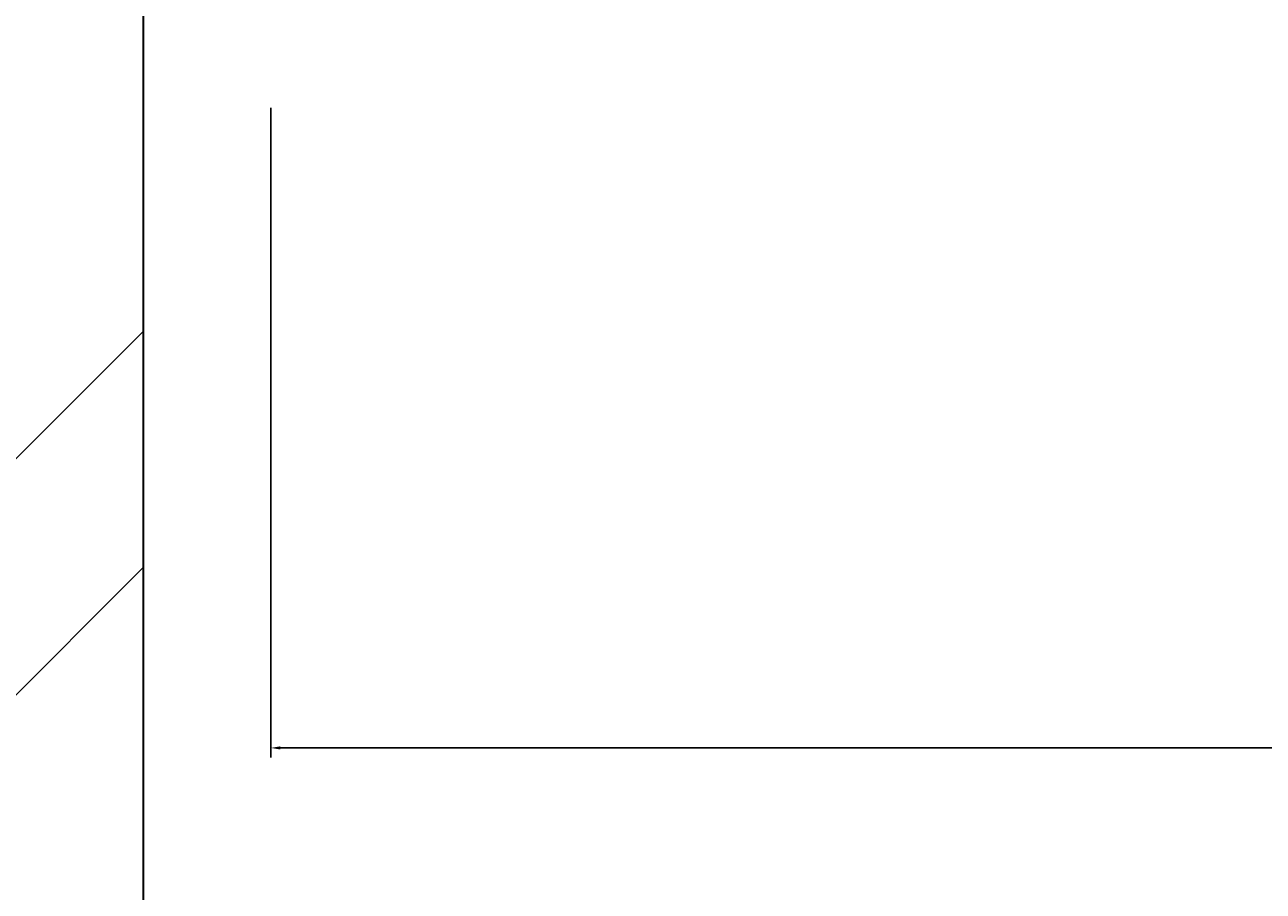
# Model space of a CAD drawing. Units: inches. Extents: x 2168 to 3056, y 1130 to 2629.
# Tile 24 of 42: x 2462 to 2485, y 2305 to 2321. Entities that reach past the tile are written whole.
import ezdxf

# ---------------------------------------------------------------- set-up
doc = ezdxf.new("R2010")
doc.units = ezdxf.units.IN
doc.layers.add('A-ANNO-DIMS', color=2, linetype='Continuous', lineweight=18)
doc.layers.add('A-WALL', color=7, linetype='Continuous', lineweight=35)
doc.layers.add('A-WALL-PATT', color=143, linetype='Continuous', lineweight=13, true_color=0x7aafdf)
doc.styles.get("Standard").update_dxf_attribs({"font": 'arial.ttf'})
doc.dimstyles.get("Standard").update_dxf_attribs({"dimtxt": 0.18, "dimasz": 0.18, "dimexe": 0.18, "dimexo": 0.0625, "dimgap": 0.09, "dimtad": 0, "dimtih": 1, "dimtoh": 1, "dimdec": 4, "dimzin": 0, "dimdsep": 46, "dimtxsty": 'Standard', "dimcen": 0.09, "dimadec": 0, "dimazin": 0, "dimtfac": 1, "dimtdec": 4, "dimtofl": 0, "dimtmove": 0, "dimatfit": 3, "dimfxl": 1, "dimtolj": 1, "dimtzin": 0, "dimarcsym": 0})

# ---------------------------------------------------------------- blocks, each defined once
blk = doc.blocks.new('*D14')
at = {"layer": 'A-ANNO-DIMS', "color": 0, "lineweight": -2, "transparency": 16777216}
for p, q in [((2466.224, 2319.873), (2466.224, 2307.523)), ((2547.772, 2319.873), (2547.772, 2307.523)), ((2466.404, 2307.703), (2506.18, 2307.703)), ((2547.592, 2307.703), (2507.815, 2307.703))]:
    blk.add_line(p, q, dxfattribs=at)
at = {"layer": 'A-ANNO-DIMS', "color": 0, "transparency": 16777216}
for points in [[(2466.404, 2307.733), (2466.404, 2307.673), (2466.224, 2307.703)], [(2547.592, 2307.733), (2547.592, 2307.673), (2547.772, 2307.703)]]:
    blk.add_solid(points, dxfattribs=at)
at = {"layer": 'Defpoints', "color": 0, "transparency": 16777216}
for p in [(2466.224, 2319.935), (2547.772, 2319.935), (2547.772, 2307.703)]:
    blk.add_point(p, dxfattribs=at)
at = {"layer": 'A-ANNO-DIMS', "color": 0, "transparency": 16777216, "insert": (2506.998, 2307.703), "char_height": 0.18, "attachment_point": 5}
blk.add_mtext('\\A1;BED 82 TYP.', dxfattribs=at)

msp = doc.modelspace()

# ---------------------------------------------------------------- hatches: boundary and pattern name
at = {"layer": 'A-WALL-PATT'}
h = msp.add_hatch(dxfattribs=at)
h.set_pattern_fill('ANSI32', color=256)
h.paths.add_polyline_path([(2463.796, 2409.389), (2467.387, 2409.389), (2467.387, 2413.889), (2454.768, 2413.889), (2454.768, 2411.639), (2454.768, 2409.389), (2459.296, 2409.389), (2459.296, 2265.389), (2455.644, 2265.389), (2455.644, 2260.889), (2467.349, 2260.889), (2467.349, 2263.139), (2467.349, 2265.389), (2463.796, 2265.389)])
h.paths.add_polyline_path([(2431.596, 2413.889), (2409.647, 2413.889), (2409.647, 2409.389), (2431.596, 2409.389), (2431.596, 2411.639)])
h.paths.add_polyline_path([(2349.647, 2413.889), (2331.796, 2413.889), (2331.796, 2362.671), (2336.296, 2362.671), (2336.296, 2409.389), (2349.647, 2409.389), (2349.647, 2411.639)])
h.paths.add_polyline_path([(2634.149, 2411.639), (2634.149, 2413.889), (2562.293, 2413.889), (2562.293, 2409.389), (2595.796, 2409.389), (2595.796, 2280.309), (2595.826, 2280.309), (2595.826, 2265.389), (2499.91, 2265.389), (2499.91, 2260.889), (2550.796, 2260.889), (2550.796, 2117.308), (2555.296, 2117.308), (2555.296, 2168.08), (2571.93, 2168.08), (2571.93, 2176.889), (2559.796, 2176.889), (2559.796, 2256.389), (2640.796, 2256.389), (2640.796, 2176.889), (2626.428, 2176.889), (2626.428, 2168.08), (2645.296, 2168.08), (2645.296, 2116.637), (2649.796, 2116.637), (2649.796, 2260.889), (2691.251, 2260.889), (2691.251, 2263.139), (2691.251, 2265.389), (2670.655, 2265.389), (2670.655, 2265.365), (2600.296, 2265.365), (2600.296, 2280.258), (2600.296, 2409.389), (2634.149, 2409.389)])
h.paths.add_polyline_path([(2600.296, 2473.889), (2612.84, 2473.889), (2612.84, 2478.389), (2572.636, 2478.389), (2572.636, 2473.889), (2595.796, 2473.889), (2595.796, 2413.889), (2600.296, 2413.889)])
h.paths.add_polyline_path([(2535.796, 2473.889), (2548.636, 2473.889), (2548.636, 2478.389), (2531.396, 2478.389), (2531.396, 2413.889), (2521.6, 2413.889), (2521.6, 2409.389), (2539.239, 2409.389), (2539.239, 2411.639), (2539.239, 2413.889), (2535.796, 2413.889)])
h.paths.add_polyline_path([(2664.796, 2478.389), (2636.84, 2478.389), (2636.84, 2473.889), (2660.296, 2473.889), (2660.296, 2413.889), (2656.165, 2413.889), (2656.165, 2409.389), (2671.684, 2409.389), (2671.684, 2411.639), (2671.684, 2413.889), (2664.796, 2413.889)])
h.paths.add_polyline_path([(2705.942, 2413.889), (2695.684, 2413.889), (2695.684, 2409.389), (2705.942, 2409.389)])
h.paths.add_polyline_path([(2741.35, 2413.889), (2728.733, 2413.889), (2728.733, 2411.639), (2728.733, 2409.389), (2732.296, 2409.389), (2732.296, 2265.389), (2725.733, 2265.389), (2725.733, 2260.889), (2740.917, 2260.889), (2740.917, 2263.139), (2740.917, 2265.389), (2736.796, 2265.389), (2736.796, 2409.389), (2741.35, 2409.389)])
h.paths.add_polyline_path([(2785.655, 2413.889), (2764.546, 2413.889), (2764.486, 2409.389), (2785.655, 2409.389), (2785.655, 2411.639)])
h.paths.add_polyline_path([(2864.296, 2413.889), (2845.655, 2413.889), (2845.655, 2409.389), (2859.796, 2409.389), (2859.796, 2368.425), (2864.296, 2368.425)])
h.paths.add_polyline_path([(2864.296, 2308.425), (2862.046, 2308.425), (2859.796, 2308.425), (2859.796, 2265.389), (2774.483, 2265.389), (2774.483, 2263.139), (2774.483, 2260.889), (2781.796, 2260.889), (2781.796, 2226.654), (2786.296, 2226.654), (2786.296, 2260.889), (2859.796, 2260.889), (2859.796, 2241.352), (2864.296, 2241.352)])
h.paths.add_polyline_path([(2864.296, 2217.352), (2862.046, 2217.352), (2859.796, 2217.352), (2859.796, 2200.889), (2786.296, 2200.889), (2786.296, 2205.931), (2784.046, 2205.931), (2781.796, 2205.931), (2781.796, 2150.974), (2786.296, 2150.974), (2786.296, 2161.889), (2859.796, 2161.889), (2859.796, 2144.419), (2864.296, 2144.419)])
h.paths.add_polyline_path([(2859.796, 2196.389), (2859.796, 2166.389), (2786.296, 2166.389), (2786.296, 2196.389)], flags=16)
h.paths.add_polyline_path([(2864.296, 2108.419), (2862.046, 2108.419), (2859.796, 2108.419), (2859.796, 2080.889), (2786.296, 2080.889), (2786.296, 2111.993), (2781.796, 2111.993), (2781.796, 2080.889), (2649.796, 2080.889), (2649.796, 2086.036), (2647.546, 2086.036), (2645.296, 2086.036), (2645.296, 2071.739), (2649.796, 2071.739), (2649.796, 2076.389), (2781.796, 2076.389), (2781.796, 2041.792), (2786.296, 2041.792), (2786.296, 2076.389), (2859.796, 2076.389), (2859.796, 2058.577), (2864.296, 2058.577)])
h.paths.add_polyline_path([(2864.296, 2022.577), (2859.796, 2022.577), (2859.796, 1992.389), (2786.296, 1992.389), (2786.296, 1999.573), (2781.796, 1999.573), (2781.796, 1848.085), (2784.046, 1848.085), (2786.296, 1848.085), (2786.296, 1851.389), (2859.796, 1851.389), (2859.796, 1838.258), (2864.296, 1838.258)], flags=17)
h.paths.add_polyline_path([(2859.796, 1987.889), (2859.796, 1855.889), (2786.296, 1855.889), (2786.296, 1987.889)], flags=16)
h.paths.add_polyline_path([(2823.046, 1987.889), (2841.421, 1921.889), (2823.046, 1855.889)], flags=0)
h.paths.add_polyline_path([(2864.296, 1814.258), (2859.796, 1814.258), (2859.796, 1791.389), (2786.296, 1791.389), (2786.296, 1825.658), (2784.046, 1825.658), (2781.796, 1825.658), (2781.796, 1791.389), (2720.155, 1791.389), (2720.155, 1791.265), (2649.796, 1791.265), (2649.796, 1806.159), (2649.796, 2038.983), (2647.546, 2038.983), (2645.296, 2038.983), (2645.296, 1783.925), (2649.796, 1783.925), (2649.796, 1786.889), (2781.796, 1786.889), (2781.796, 1746.789), (2786.296, 1746.789), (2786.296, 1786.889), (2859.796, 1786.889), (2859.796, 1770.083), (2864.296, 1770.083)])
h.paths.add_polyline_path([(2864.296, 1734.083), (2862.046, 1734.083), (2859.796, 1734.083), (2859.796, 1705.889), (2786.296, 1705.889), (2786.296, 1714.166), (2781.796, 1714.166), (2781.796, 1660.527), (2786.296, 1660.527), (2786.296, 1666.889), (2859.796, 1666.889), (2859.796, 1648.342), (2864.296, 1648.342)])
h.paths.add_polyline_path([(2786.296, 1701.389), (2859.796, 1701.389), (2859.796, 1671.389), (2786.296, 1671.389)], flags=16)
h.paths.add_polyline_path([(2649.796, 1756.576), (2647.546, 1756.576), (2645.296, 1756.576), (2645.296, 1606.889), (2555.296, 1606.889), (2555.296, 1749.513), (2553.046, 1749.513), (2550.796, 1749.513), (2550.796, 1606.889), (2503.006, 1606.889), (2503.006, 1604.639), (2503.006, 1602.389), (2595.796, 1602.389), (2595.849, 1602.389), (2595.849, 1587.495), (2595.796, 1458.389), (2561.502, 1458.389), (2561.502, 1456.139), (2561.502, 1453.889), (2595.796, 1453.889), (2595.796, 1381.889), (2573.438, 1381.889), (2573.438, 1377.389), (2613.01, 1377.389), (2613.01, 1379.639), (2613.01, 1381.889), (2600.296, 1381.889), (2600.296, 1453.889), (2634.327, 1453.889), (2634.327, 1458.389), (2600.296, 1458.389), (2600.296, 1602.389), (2670.655, 1602.389), (2694.095, 1602.389), (2694.095, 1606.889), (2649.796, 1606.889)])
h.paths.add_polyline_path([(2736.796, 1602.389), (2741.562, 1602.389), (2741.562, 1606.889), (2726.203, 1606.889), (2726.203, 1604.639), (2726.203, 1602.389), (2732.296, 1602.389), (2732.296, 1458.389), (2727.899, 1458.389), (2727.899, 1453.889), (2740.821, 1453.889), (2740.821, 1456.139), (2740.821, 1458.389), (2736.796, 1458.389)])
h.paths.add_polyline_path([(2859.796, 1606.889), (2786.296, 1606.889), (2786.296, 1637.334), (2784.046, 1637.334), (2781.796, 1637.334), (2781.796, 1606.889), (2775.612, 1606.889), (2775.612, 1602.389), (2859.796, 1602.389)])
h.paths.add_polyline_path([(2864.296, 1624.342), (2862.046, 1624.342), (2859.796, 1624.342), (2859.796, 1570.39), (2864.296, 1570.39)])
h.paths.add_polyline_path([(2864.296, 1510.39), (2862.046, 1510.39), (2859.796, 1510.39), (2859.796, 1458.389), (2846.735, 1458.389), (2846.735, 1456.139), (2846.735, 1453.889), (2864.296, 1453.889)])
h.paths.add_polyline_path([(2786.735, 1458.389), (2765.444, 1458.389), (2765.444, 1453.889), (2786.735, 1453.889)])
h.paths.add_polyline_path([(2706.004, 1458.389), (2695.36, 1458.389), (2695.36, 1453.889), (2706.004, 1453.889), (2706.004, 1456.139)])
h.paths.add_polyline_path([(2671.36, 1456.139), (2671.36, 1458.389), (2655.986, 1458.389), (2655.986, 1456.139), (2655.986, 1453.889), (2660.296, 1453.889), (2660.296, 1381.889), (2637.01, 1381.889), (2637.01, 1377.389), (2664.796, 1377.389), (2664.796, 1453.889), (2671.36, 1453.889)], flags=17)
h.paths.add_polyline_path([(2539.829, 1458.389), (2520.237, 1458.389), (2520.237, 1453.889), (2531.296, 1453.889), (2531.296, 1377.389), (2546.449, 1377.389), (2546.449, 1379.639), (2546.449, 1381.889), (2535.796, 1381.889), (2535.796, 1453.889), (2539.829, 1453.889)], flags=17)
h.paths.add_polyline_path([(2496.237, 1458.389), (2489.13, 1458.389), (2489.13, 1453.889), (2496.237, 1453.889), (2496.237, 1456.139)])
h.paths.add_polyline_path([(2467.433, 1456.139), (2467.433, 1458.389), (2463.796, 1458.389), (2463.796, 1602.389), (2468.242, 1602.389), (2468.242, 1605.7), (2468.242, 1606.889), (2454.602, 1606.889), (2454.602, 1602.389), (2459.296, 1602.389), (2459.296, 1458.389), (2454.24, 1458.389), (2454.24, 1453.889), (2467.433, 1453.889)])
h.paths.add_polyline_path([(2431.601, 1456.139), (2431.601, 1458.389), (2411.386, 1458.389), (2411.386, 1453.889), (2431.601, 1453.889)])
h.paths.add_polyline_path([(2351.386, 1458.389), (2336.296, 1458.389), (2336.296, 1490.693), (2334.046, 1490.693), (2331.796, 1490.693), (2331.796, 1453.889), (2351.386, 1453.889), (2351.386, 1456.139)])
h.paths.add_polyline_path([(2336.296, 1629.705), (2331.796, 1629.705), (2331.796, 1552.317), (2336.296, 1552.317), (2336.296, 1602.389), (2406.655, 1602.389), (2423.472, 1602.389), (2423.472, 1606.889), (2418.796, 1606.889), (2418.796, 1643.678), (2416.546, 1643.678), (2414.296, 1643.678), (2414.296, 1606.889), (2336.296, 1606.889)])
h.paths.add_polyline_path([(2418.796, 1714.384), (2414.296, 1714.384), (2414.296, 1705.889), (2336.296, 1705.889), (2336.296, 1731.324), (2334.046, 1731.324), (2331.796, 1731.324), (2331.796, 1653.705), (2334.046, 1653.705), (2336.296, 1653.705), (2336.296, 1666.889), (2414.296, 1666.889), (2414.296, 1663.589), (2418.796, 1663.589)])
h.paths.add_polyline_path([(2336.296, 1701.389), (2414.296, 1701.389), (2414.296, 1671.389), (2336.296, 1671.389)], flags=16)
h.paths.add_polyline_path([(2555.296, 2040.059), (2550.796, 2040.059), (2550.796, 1791.389), (2550.561, 1791.205), (2480.202, 1791.205), (2418.796, 1791.389), (2418.796, 1825.448), (2416.546, 1825.448), (2414.296, 1825.448), (2414.296, 1791.389), (2336.296, 1791.389), (2336.296, 1806.409), (2331.796, 1806.409), (2331.796, 1767.324), (2336.296, 1767.324), (2336.296, 1786.889), (2414.296, 1786.889), (2414.296, 1745.457), (2418.796, 1745.457), (2418.796, 1786.889), (2550.796, 1786.889), (2550.796, 1783.011), (2555.296, 1783.011)])
h.paths.add_polyline_path([(2418.796, 1923.389), (2423.207, 1923.389), (2423.207, 1925.639), (2423.207, 1927.889), (2418.796, 1927.889), (2418.796, 2000.048), (2414.296, 2000.048), (2414.296, 1992.389), (2336.296, 1992.389), (2336.296, 1987.889), (2414.296, 1987.889), (2414.296, 1855.889), (2336.296, 1855.889), (2336.296, 1851.389), (2414.296, 1851.389), (2414.296, 1846.759), (2418.796, 1846.759)], flags=17)
h.paths.add_polyline_path([(2336.296, 2019.294), (2334.046, 2019.294), (2331.796, 2019.294), (2331.796, 1830.409), (2336.296, 1830.409)], flags=17)
h.paths.add_polyline_path([(2550.796, 1927.889), (2453.541, 1927.889), (2453.541, 1925.639), (2453.541, 1923.389), (2550.796, 1923.389)], flags=17)
h.paths.add_polyline_path([(2744.987, 1927.889), (2649.796, 1927.889), (2649.796, 1923.389), (2744.987, 1923.389), (2744.987, 1925.639)], flags=17)
h.paths.add_polyline_path([(2555.296, 2086.458), (2553.046, 2086.458), (2550.796, 2086.458), (2550.796, 2080.889), (2418.796, 2080.889), (2336.296, 2080.889), (2336.296, 2115.399), (2334.046, 2115.399), (2331.796, 2115.399), (2331.796, 2055.294), (2336.296, 2055.294), (2336.296, 2076.389), (2550.796, 2076.389), (2550.796, 2071.538), (2555.296, 2071.538)])
h.paths.add_polyline_path([(2418.796, 2121.389), (2414.296, 2121.389), (2414.296, 2080.889), (2418.796, 2080.889)])
h.paths.add_polyline_path([(2418.796, 2076.389), (2414.296, 2076.389), (2414.296, 2035.123), (2418.796, 2035.123)])
h.paths.add_polyline_path([(2422.868, 2263.139), (2422.868, 2265.389), (2406.655, 2265.389), (2406.655, 2265.359), (2336.296, 2265.359), (2336.296, 2280.252), (2336.296, 2302.671), (2334.046, 2302.671), (2331.796, 2302.671), (2331.796, 2246.853), (2336.296, 2246.853), (2336.296, 2260.889), (2414.296, 2260.889), (2414.296, 2223.996), (2418.796, 2223.996), (2418.796, 2260.889), (2422.868, 2260.889)])
h.paths.add_polyline_path([(2418.796, 2204.783), (2416.546, 2204.783), (2414.296, 2204.783), (2414.296, 2200.889), (2336.296, 2200.889), (2336.296, 2220.853), (2331.796, 2220.853), (2331.796, 2151.399), (2336.296, 2151.399), (2336.296, 2161.889), (2414.296, 2161.889), (2414.296, 2153.726), (2418.796, 2153.726)])
h.paths.add_polyline_path([(2414.296, 2196.389), (2414.296, 2166.389), (2336.296, 2166.389), (2336.296, 2196.389)], flags=16)
h.paths.add_polyline_path([(2375.296, 2181.389), (2336.296, 2166.389), (2336.296, 2196.389)], flags=0)
h.paths.add_polyline_path([(2809.595, 2172.34), (2838.804, 2172.34), (2838.804, 2190.997), (2809.595, 2190.997)], flags=8)
h.paths.add_polyline_path([(2849.75, 1919.585), (2849.75, 1952.672), (2831.093, 1952.672), (2831.093, 1919.585)], flags=8)
h.paths.add_polyline_path([(2808.875, 1901.967), (2808.875, 1937.85), (2790.149, 1937.85), (2790.149, 1901.967)], flags=8)
h.paths.add_polyline_path([(2806.285, 1671.896), (2835.493, 1671.896), (2835.493, 1690.553), (2806.285, 1690.553)], flags=8)
h.paths.add_polyline_path([(2353.186, 1676.549), (2382.395, 1676.549), (2382.395, 1695.207), (2353.186, 1695.207)], flags=8)
h.paths.add_polyline_path([(2360.083, 1832.308), (2389.241, 1832.308), (2389.241, 1850.966), (2360.083, 1850.966)], flags=25)
h.paths.add_polyline_path([(2354.822, 2167.823), (2384.031, 2167.823), (2384.031, 2186.481), (2354.822, 2186.481)], flags=8)

# ---------------------------------------------------------------- linework, layer by layer
at = {"layer": 'A-WALL'}
msp.add_line((2463.796, 2409.389), (2463.796, 2265.389), dxfattribs=at)

# ---------------------------------------------------------------- dimensions: what is measured, and where the dimension line sits
at = {"layer": 'A-ANNO-DIMS'}
dim = msp.add_linear_dim(base=(2547.772, 2307.703), p1=(2466.224, 2319.935), p2=(2547.772, 2319.935), text='BED <> TYP.', dimstyle='Standard', override={"dimdec": 0, "dimlfac": 1, "dimrnd": 0, "dimzin": 0, "dimdsep": 46, "dimlunit": 2}, dxfattribs=at)
dim.commit()
dim.dimension.update_dxf_attribs({"geometry": '*D14', "text_midpoint": (2506.998, 2307.703)})

doc.saveas('drawing.dxf')
